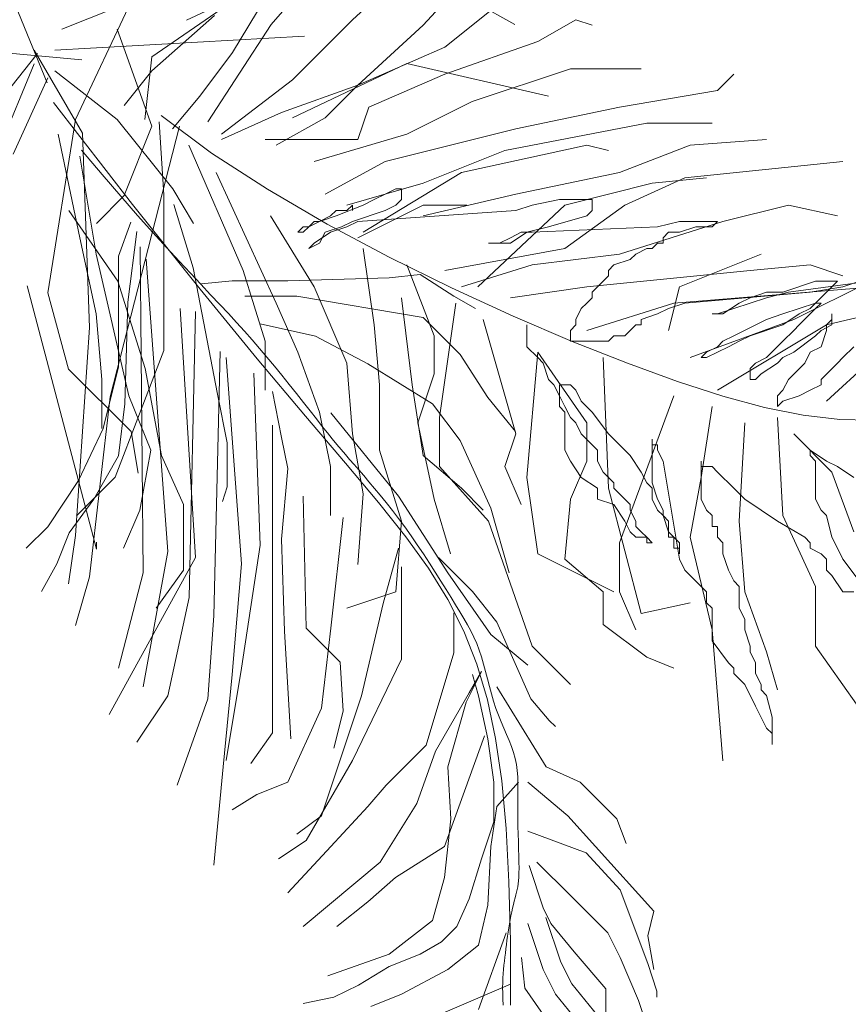
# Model space of a CAD drawing. Units: millimetres. Extents: x 595116 to 630915, y 909473 to 920225.
# Tile 58 of 134: x 629601.67 to 629606.022, y 919290.711 to 919295.882. Entities that reach past the tile are written whole.
import ezdxf

# ---------------------------------------------------------------- set-up
doc = ezdxf.new("R2010")
doc.units = ezdxf.units.MM
doc.layers.add('Dimension', color=3, linetype='Continuous', lineweight=18)
doc.layers.add('L-PLNT', color=85, linetype='Continuous', lineweight=13)
doc.styles.get("Standard").update_dxf_attribs({"font": 'arial.ttf'})
doc.dimstyles.new('ISO-25', dxfattribs={"dimtxt": 9, "dimasz": 6, "dimexe": 1.25, "dimexo": 0.625, "dimtad": 1, "dimlunit": 4, "dimtxsty": 'Standard', "dimcen": 2.5, "dimadec": 0, "dimazin": 0, "dimtfac": 1, "dimtmove": 0, "dimatfit": 3, "dimfxl": 1, "dimarcsym": 0})

# ---------------------------------------------------------------- blocks, each defined once
blk = doc.blocks.new('A$C4FB75ABC')
for p, q in [((2.6324, 2.4053), (2.7073, 2.2214)), ((3.0207, 2.3031), (3.1093, 2.4053)), ((3.1344, 2.3096), (3.2259, 2.3934)), ((3.2335, 2.302), (3.3174, 2.3934)), ((2.9022, 2.3089), (3.0036, 2.3566)), ((2.7277, 2.2964), (2.8733, 2.3546)), ((2.8539, 2.2576), (2.9801, 2.3449)), ((2.8248, 2.3352), (2.7471, 2.1703)), ((2.9666, 2.2638), (3.0123, 2.3401)), ((3.264, 2.2715), (3.3403, 2.3324)), ((3.3079, 2.3327), (3.3615, 2.3029)), ((2.8539, 2.2382), (2.9413, 2.3158)), ((2.9321, 2.167), (3.0207, 2.3031)), ((3.0505, 2.2257), (3.1344, 2.3096)), ((3.142, 2.2181), (3.2335, 2.302)), ((3.3937, 2.2791), (3.447, 2.3096)), ((3.447, 2.3096), (3.4699, 2.302)), ((2.8054, 2.2964), (2.8539, 2.1606)), ((2.7559, 2.2536), (2.4852, 2.2785)), ((2.718, 2.2673), (3.0675, 2.2867)), ((3.264, 2.2334), (3.3937, 2.2791)), ((2.6937, 2.2623), (2.4825, 1.9967)), ((2.6889, 2.2673), (2.7568, 2.1509)), ((2.9208, 2.2029), (2.9666, 2.2638)), ((3.142, 2.2181), (3.264, 2.2715)), ((2.6889, 2.2479), (2.6404, 2.1315)), ((2.8442, 2.1703), (2.8539, 2.2576)), ((3.0505, 2.1724), (3.2106, 2.2486)), ((3.2106, 2.2486), (3.4089, 2.2029)), ((2.718, 2.2382), (2.8054, 2.1703)), ((2.8151, 2.1897), (2.8539, 2.2382)), ((3.1572, 2.1876), (3.264, 2.2334)), ((3.3021, 2.1952), (3.4394, 2.241)), ((3.4394, 2.241), (3.5385, 2.241)), ((3.6453, 2.2105), (3.6682, 2.2334)), ((2.7083, 2.2285), (2.6598, 2.1218)), ((2.9513, 2.1495), (3.0505, 2.2257)), ((3.0352, 2.18), (3.142, 2.2181)), ((3.0962, 2.1724), (3.142, 2.2181)), ((3.508, 2.1876), (3.6453, 2.2105)), ((2.7162, 2.1941), (2.8268, 2.0511)), ((2.8827, 2.1571), (2.9208, 2.2029)), ((3.2106, 2.1495), (3.3021, 2.1952)), ((2.9513, 2.1419), (3.0352, 2.18)), ((3.142, 2.1419), (3.1572, 2.1876)), ((3.3631, 2.1571), (3.508, 2.1876)), ((2.7471, 2.1703), (2.7083, 1.9277)), ((2.8054, 2.1703), (2.883, 2.0733)), ((2.864, 2.167), (2.8708, 2.0648)), ((2.9375, 2.1232), (2.8667, 2.1755)), ((3.0276, 2.1343), (3.0962, 2.1724)), ((3.3479, 2.1266), (3.5462, 2.1648)), ((3.5462, 2.1648), (3.6377, 2.1648)), ((2.7225, 2.1495), (2.753, 2.0047)), ((2.7568, 2.1509), (2.7666, 1.8792)), ((2.8927, 2.1606), (2.7957, 1.7822)), ((2.8539, 2.1606), (2.8151, 2.0636)), ((3.081, 2.1114), (3.2106, 2.1495)), ((3.1801, 2.1114), (3.3631, 2.1571)), ((3.0123, 2.1419), (3.142, 2.1419)), ((3.6072, 2.1343), (3.714, 2.1419)), ((2.7555, 2.1274), (2.7844, 2.0931)), ((2.9056, 2.1343), (2.9818, 1.9589)), ((3.0158, 2.0725), (2.9375, 2.1232)), ((3.2335, 2.0809), (3.3479, 2.1266)), ((3.2869, 2.0961), (3.4623, 2.1343)), ((3.4623, 2.1343), (3.4928, 2.1266)), ((3.508, 2.0961), (3.6072, 2.1343)), ((2.753, 2.119), (2.7759, 1.9818)), ((3.0962, 2.0657), (3.1801, 2.1114)), ((3.5996, 2.0885), (3.8207, 2.1114)), ((2.9437, 2.0961), (3.0276, 1.9132)), ((3.1496, 2.0123), (3.2869, 2.0961)), ((3.3631, 2.0657), (3.508, 2.0961)), ((2.7844, 2.0931), (2.8104, 2.0628)), ((3.1267, 2.0504), (3.2335, 2.0809)), ((3.4318, 2.0504), (3.5538, 2.0809)), ((3.5157, 2.0504), (3.5996, 2.0885)), ((3.5538, 2.0809), (3.6301, 2.0885)), ((2.883, 2.0733), (2.9122, 2.0248)), ((3.0992, 2.0238), (3.0158, 2.0725)), ((3.1954, 2.0733), (3.1801, 2.0657)), ((3.203, 2.0733), (3.1954, 2.0733)), ((3.203, 2.058), (3.203, 2.0733)), ((2.8151, 2.0636), (2.7763, 2.0248)), ((2.8104, 2.0628), (2.8339, 2.0359)), ((2.8708, 2.0648), (2.8708, 1.8469)), ((3.1649, 2.058), (3.1496, 2.0504)), ((3.1801, 2.0657), (3.1649, 2.058)), ((3.1954, 2.0504), (3.203, 2.058)), ((3.2335, 2.0352), (3.3631, 2.0657)), ((3.4242, 2.058), (3.386, 2.0504)), ((3.4699, 2.058), (3.4242, 2.058)), ((3.4699, 2.0428), (3.4699, 2.058)), ((2.7378, 2.0428), (2.8064, 1.9437)), ((2.8268, 2.0511), (2.9214, 1.9326)), ((2.8844, 2.0512), (2.9117, 1.9627)), ((3.1039, 2.0352), (3.1115, 2.0428)), ((3.1496, 2.0504), (3.1115, 2.0352)), ((3.1115, 2.0428), (3.1267, 2.0428)), ((3.1267, 2.0428), (3.1344, 2.0504)), ((3.1344, 2.0504), (3.1344, 2.0428)), ((3.1344, 2.0275), (3.1801, 2.0428)), ((3.142, 2.0047), (3.2335, 2.0504)), ((3.3631, 2.0428), (3.142, 2.0275)), ((3.1801, 2.0428), (3.1954, 2.0504)), ((3.2335, 2.0504), (3.2945, 2.0504)), ((3.3098, 1.9361), (3.4318, 2.0504)), ((3.386, 2.0504), (3.3631, 2.0428)), ((3.4318, 1.9894), (3.5157, 2.0504)), ((3.4623, 2.0352), (3.4699, 2.0428)), ((3.6529, 2.0275), (3.7445, 2.0504)), ((3.7445, 2.0504), (3.8131, 2.0352)), ((2.8244, 2.0263), (2.8071, 1.979)), ((2.8339, 2.0359), (2.8551, 2.0121)), ((3.02, 2.0352), (3.081, 1.9361)), ((3.0734, 2.0199), (3.081, 2.0275)), ((3.0886, 2.0275), (3.0734, 2.0199)), ((3.081, 2.0275), (3.0886, 2.0275)), ((3.1115, 2.0352), (3.0886, 2.0275)), ((3.0886, 2.0275), (3.1039, 2.0352)), ((3.1191, 2.0199), (3.1344, 2.0275)), ((3.142, 2.0275), (3.1267, 2.0199)), ((3.4089, 2.0199), (3.4623, 2.0352)), ((3.508, 1.9818), (3.6529, 2.0275)), ((3.5919, 2.0275), (3.5614, 2.0199)), ((3.6453, 2.0275), (3.5919, 2.0275)), ((3.6377, 2.0199), (3.6453, 2.0275)), ((2.833, 2.0134), (2.8201, 1.9144)), ((2.8551, 2.0121), (2.8744, 1.9909)), ((3.0581, 2.0123), (3.0657, 2.0199)), ((3.0657, 2.0123), (3.0581, 2.0123)), ((3.0734, 2.0199), (3.0657, 2.0123)), ((3.0657, 2.0199), (3.0734, 2.0199)), ((3.1039, 2.0123), (3.081, 1.9971)), ((3.0886, 1.9971), (3.0962, 2.0123)), ((3.0962, 2.0123), (3.1191, 2.0199)), ((3.1858, 1.9776), (3.0992, 2.0238)), ((3.1267, 2.0199), (3.1039, 2.0123)), ((3.3708, 2.0123), (3.3555, 2.0047)), ((3.3555, 1.9971), (3.3784, 2.0123)), ((3.386, 2.0123), (3.3708, 2.0123)), ((3.3784, 2.0123), (3.4089, 2.0199)), ((3.5614, 2.0199), (3.386, 2.0123)), ((3.5691, 2.0047), (3.5767, 2.0123)), ((3.5767, 2.0123), (3.5919, 2.0123)), ((3.5919, 2.0123), (3.6148, 2.0199)), ((3.6148, 2.0199), (3.6377, 2.0199)), ((2.753, 2.0047), (2.7759, 1.898)), ((3.3555, 2.0047), (3.3403, 1.9971)), ((3.5691, 1.9971), (3.5691, 2.0047)), ((2.8373, 1.9919), (2.8416, 1.5357)), ((2.8744, 1.9909), (2.8918, 1.9721)), ((3.081, 1.9971), (3.0734, 1.9894)), ((3.0734, 1.9894), (3.0886, 1.9971)), ((3.1496, 1.9894), (3.1649, 1.8827)), ((3.264, 1.9589), (3.4318, 1.9894)), ((3.3403, 1.9971), (3.325, 1.9971)), ((3.325, 1.9971), (3.3555, 1.9971)), ((3.5309, 1.9818), (3.5462, 1.9894)), ((3.5462, 1.9894), (3.5538, 1.9894)), ((3.5538, 1.9894), (3.5614, 1.9971)), ((3.5614, 1.9971), (3.5691, 1.9971)), ((2.7759, 1.9818), (2.8217, 1.7836)), ((2.8071, 1.979), (2.8071, 1.9015)), ((2.8459, 1.9747), (2.876, 1.5659)), ((2.8918, 1.9721), (2.9078, 1.955)), ((3.2732, 1.9345), (3.1858, 1.9776)), ((3.386, 1.9666), (3.508, 1.9818)), ((3.5004, 1.9666), (3.5233, 1.9742)), ((3.5233, 1.9742), (3.5309, 1.9818)), ((3.5919, 1.9361), (3.7063, 1.9818)), ((2.9117, 1.9627), (2.9458, 1.7856)), ((2.9818, 1.9589), (3.0123, 1.8599)), ((3.2106, 1.9666), (3.2488, 1.8675)), ((3.2869, 1.9361), (3.386, 1.9666)), ((3.4623, 1.9361), (3.6911, 1.9589)), ((3.4928, 1.9589), (3.5004, 1.9666)), ((3.4928, 1.9513), (3.4928, 1.9589)), ((3.6911, 1.9589), (3.775, 1.9666)), ((3.7521, 1.8903), (3.8894, 1.9589)), ((3.775, 1.9666), (3.8207, 1.9513)), ((2.8064, 1.9437), (2.8446, 1.8217)), ((2.9078, 1.955), (2.9225, 1.9395)), ((2.9234, 1.9402), (2.9664, 1.9445)), ((2.9664, 1.9445), (3.0439, 1.9445)), ((3.0439, 1.9445), (3.186, 1.9488)), ((3.186, 1.9488), (3.2291, 1.9531)), ((3.2291, 1.9531), (3.2764, 1.923)), ((3.4699, 1.9285), (3.4852, 1.9437)), ((3.4852, 1.9437), (3.4928, 1.9513)), ((3.7826, 1.9437), (3.7368, 1.9285)), ((3.7445, 1.9285), (3.9122, 1.9513)), ((3.7826, 1.9132), (3.8131, 1.9437)), ((3.8131, 1.9437), (3.7826, 1.9437)), ((3.7978, 1.8827), (4.0495, 1.9437)), ((3.8665, 1.9513), (3.8207, 1.9361)), ((2.6792, 1.9375), (2.7763, 1.5688)), ((2.9214, 1.9326), (3.0014, 1.8351)), ((2.9225, 1.9395), (2.9361, 1.925)), ((3.081, 1.9361), (3.1267, 1.8294)), ((3.3593, 1.8951), (3.2732, 1.9345)), ((3.3555, 1.9208), (3.4623, 1.9361)), ((3.5767, 1.8751), (3.5919, 1.9361)), ((3.5843, 1.9132), (3.8665, 1.9361)), ((3.8207, 1.9361), (3.775, 1.9285)), ((2.7083, 1.9277), (2.7374, 1.821)), ((2.9361, 1.925), (2.9489, 1.9114)), ((2.9837, 1.923), (3.0569, 1.923)), ((3.0569, 1.923), (3.2334, 1.8929)), ((3.203, 1.9208), (3.2182, 1.7989)), ((3.2764, 1.923), (3.3066, 1.9058)), ((3.4623, 1.9132), (3.4699, 1.9208)), ((3.4699, 1.9208), (3.4699, 1.9285)), ((3.775, 1.9285), (3.5996, 1.9132)), ((3.6453, 1.898), (3.714, 1.9208)), ((3.6911, 1.9208), (3.6758, 1.9132)), ((3.714, 1.9285), (3.6911, 1.9208)), ((3.7368, 1.9285), (3.714, 1.9285)), ((3.714, 1.9208), (3.7445, 1.9285)), ((2.8071, 1.9015), (2.8071, 1.8241)), ((2.8201, 1.9144), (2.8158, 1.7724)), ((2.8933, 1.9058), (2.9148, 1.5573)), ((2.9148, 1.9015), (2.9062, 1.5013)), ((2.9489, 1.9114), (2.9609, 1.8985)), ((3.0276, 1.9132), (3.0581, 1.8446)), ((3.2793, 1.9132), (3.2564, 1.7531)), ((3.447, 1.8903), (3.4547, 1.9056)), ((3.4547, 1.9056), (3.4623, 1.9132)), ((3.4623, 1.8751), (3.5843, 1.9132)), ((3.5767, 1.9056), (3.5614, 1.898)), ((3.5996, 1.9132), (3.5767, 1.9056)), ((3.6758, 1.9132), (3.6529, 1.898)), ((3.7368, 1.898), (3.7826, 1.9132)), ((3.7597, 1.8827), (3.7826, 1.9056)), ((3.775, 1.9056), (3.7597, 1.898)), ((3.7826, 1.9132), (3.775, 1.9056)), ((3.7826, 1.9056), (3.7902, 1.9132)), ((3.7902, 1.9132), (3.7826, 1.9132)), ((2.7759, 1.898), (2.7836, 1.8065)), ((2.9609, 1.8985), (2.9724, 1.8861)), ((3.2334, 1.8929), (3.285, 1.8413)), ((3.3174, 1.8903), (3.3631, 1.7303)), ((3.4421, 1.8597), (3.3593, 1.8951)), ((3.447, 1.8827), (3.447, 1.8903)), ((3.5614, 1.898), (3.5385, 1.8903)), ((3.5385, 1.8903), (3.5385, 1.8827)), ((3.6072, 1.837), (3.7521, 1.8903)), ((3.6529, 1.898), (3.6377, 1.898)), ((3.6377, 1.898), (3.6453, 1.898)), ((3.6682, 1.8675), (3.714, 1.8903)), ((3.714, 1.8903), (3.7368, 1.898)), ((3.7597, 1.898), (3.7368, 1.8827)), ((3.7978, 1.8827), (3.8055, 1.8903)), ((3.8055, 1.8903), (3.8055, 1.898)), ((3.8055, 1.898), (3.8055, 1.8827)), ((2.7666, 1.8792), (2.7471, 1.5882)), ((2.9724, 1.8861), (2.9834, 1.874)), ((2.9834, 1.874), (2.994, 1.862)), ((3.0052, 1.8843), (3.0827, 1.8671)), ((3.1649, 1.8827), (3.1725, 1.7989)), ((3.3784, 1.8827), (3.3784, 1.8522)), ((3.4394, 1.8751), (3.447, 1.8827)), ((3.4394, 1.8599), (3.4394, 1.8751)), ((3.5233, 1.8751), (3.5157, 1.8675)), ((3.5309, 1.8827), (3.5233, 1.8751)), ((3.5385, 1.8827), (3.5309, 1.8827)), ((3.6453, 1.7913), (3.7978, 1.8827)), ((3.7368, 1.8827), (3.6911, 1.8675)), ((3.7368, 1.8599), (3.7521, 1.8751)), ((3.7521, 1.8751), (3.7597, 1.8827)), ((3.7902, 1.8751), (3.7826, 1.8675)), ((3.8055, 1.8827), (3.7902, 1.8751)), ((3.7902, 1.8522), (3.7978, 1.8751)), ((3.7978, 1.8751), (3.7978, 1.8827)), ((2.994, 1.862), (3.0045, 1.8499)), ((3.0123, 1.8599), (3.0123, 1.7913)), ((3.0827, 1.8671), (3.1559, 1.8284)), ((3.2488, 1.8675), (3.2488, 1.8141)), ((3.4928, 1.8599), (3.4394, 1.8599)), ((3.5004, 1.8675), (3.4928, 1.8599)), ((3.5157, 1.8675), (3.5004, 1.8675)), ((3.6453, 1.8522), (3.6529, 1.8599)), ((3.6529, 1.8599), (3.6682, 1.8675)), ((3.6758, 1.8599), (3.6606, 1.8522)), ((3.6911, 1.8675), (3.6758, 1.8599)), ((3.714, 1.837), (3.7368, 1.8599)), ((3.7826, 1.8675), (3.7521, 1.8446)), ((3.7978, 1.776), (3.897, 1.8675)), ((2.8708, 1.8469), (2.8027, 1.6699)), ((3.0045, 1.8499), (3.0149, 1.8377)), ((3.3784, 1.8522), (3.3937, 1.837)), ((3.5192, 1.829), (3.4421, 1.8597)), ((3.6606, 1.8522), (3.6301, 1.837)), ((3.6301, 1.8446), (3.6453, 1.8522)), ((3.775, 1.8446), (3.7902, 1.8522)), ((3.836, 1.8522), (3.8207, 1.837)), ((2.9492, 1.8456), (2.9406, 1.4755)), ((2.9578, 1.837), (2.9794, 1.5486)), ((3.0014, 1.8351), (3.0686, 1.7552)), ((3.0149, 1.8377), (3.0253, 1.8251)), ((3.0581, 1.8446), (3.0886, 1.7608)), ((3.285, 1.8413), (3.3238, 1.781)), ((3.3937, 1.8446), (3.3784, 1.6693)), ((3.3937, 1.8446), (3.4623, 1.7455)), ((3.3937, 1.837), (3.4013, 1.8294)), ((3.4852, 1.837), (3.4928, 1.6541)), ((3.6224, 1.837), (3.6301, 1.8446)), ((3.6301, 1.837), (3.6224, 1.837)), ((3.6987, 1.8294), (3.714, 1.837)), ((3.7368, 1.837), (3.7292, 1.8294)), ((3.7521, 1.8446), (3.7368, 1.837)), ((3.7673, 1.8294), (3.775, 1.8446)), ((3.8207, 1.837), (3.8131, 1.8294)), ((2.7374, 1.821), (2.8248, 1.7337)), ((2.8071, 1.8241), (2.7856, 1.738)), ((2.8446, 1.8217), (2.8674, 1.6998)), ((3.0253, 1.8251), (3.0358, 1.8122)), ((3.1267, 1.8294), (3.1344, 1.7303)), ((3.1559, 1.8284), (3.2463, 1.7724)), ((3.4013, 1.8294), (3.4089, 1.8065)), ((3.5892, 1.8034), (3.5192, 1.829)), ((3.6911, 1.8217), (3.6987, 1.8294)), ((3.6911, 1.8065), (3.6911, 1.8217)), ((3.7292, 1.8294), (3.7063, 1.8141)), ((3.7445, 1.8065), (3.7673, 1.8294)), ((3.8131, 1.8294), (3.7902, 1.8065)), ((2.7836, 1.8065), (2.7836, 1.7379)), ((2.9966, 1.8154), (3.0052, 1.5745)), ((3.0358, 1.8122), (3.0461, 1.7993)), ((3.2488, 1.8141), (3.2259, 1.7455)), ((3.4089, 1.8065), (3.4165, 1.7989)), ((3.6987, 1.8065), (3.6911, 1.8065)), ((3.7063, 1.8141), (3.6987, 1.8065)), ((3.7368, 1.7913), (3.7445, 1.8065)), ((3.7902, 1.8065), (3.7902, 1.7989)), ((3.0461, 1.7993), (3.0562, 1.7866)), ((3.1725, 1.7989), (3.1725, 1.7074)), ((3.2182, 1.7989), (3.2335, 1.6998)), ((3.4165, 1.7989), (3.4242, 1.7836)), ((3.4242, 1.7684), (3.4242, 1.7989)), ((3.4242, 1.7989), (3.4394, 1.7989)), ((3.4394, 1.7989), (3.447, 1.7913)), ((3.447, 1.7913), (3.4547, 1.776)), ((3.6527, 1.7828), (3.5892, 1.8034)), ((3.7292, 1.7836), (3.7368, 1.7913)), ((3.775, 1.7913), (3.7597, 1.7836)), ((3.7902, 1.7989), (3.775, 1.7913)), ((2.7957, 1.7822), (2.7666, 1.53)), ((2.8217, 1.7836), (2.8522, 1.7074)), ((2.9458, 1.7856), (2.9594, 1.7175)), ((3.0224, 1.7896), (3.0353, 1.7251)), ((3.0562, 1.7866), (3.0659, 1.7741)), ((3.3238, 1.781), (3.3625, 1.7337)), ((3.4242, 1.7836), (3.4318, 1.7684)), ((3.5843, 1.7836), (3.508, 1.5778)), ((3.7109, 1.7672), (3.6527, 1.7828)), ((3.7292, 1.7684), (3.7292, 1.7836)), ((3.7597, 1.7836), (3.7368, 1.776)), ((2.8158, 1.7724), (2.8071, 1.6993)), ((3.0659, 1.7741), (3.0752, 1.7623)), ((3.2463, 1.7724), (3.285, 1.7208)), ((3.4318, 1.7608), (3.4242, 1.7684)), ((3.4318, 1.7684), (3.4394, 1.7531)), ((3.4547, 1.776), (3.4699, 1.7608)), ((3.6377, 1.7684), (3.6224, 1.6693)), ((3.7651, 1.7564), (3.7109, 1.7672)), ((3.7368, 1.776), (3.7292, 1.7684)), ((3.0686, 1.7552), (3.1246, 1.6894)), ((3.0752, 1.7623), (3.084, 1.7511)), ((3.084, 1.7511), (3.0921, 1.7408)), ((3.0886, 1.7608), (3.1039, 1.6845)), ((3.1042, 1.7595), (3.1989, 1.6433)), ((3.2564, 1.7531), (3.2564, 1.6845)), ((3.4318, 1.7074), (3.4318, 1.7608)), ((3.4394, 1.7531), (3.447, 1.7455)), ((3.4699, 1.7608), (3.4928, 1.7303)), ((3.7292, 1.7531), (3.7368, 1.6159)), ((3.8165, 1.7504), (3.7651, 1.7564)), ((3.8664, 1.749), (3.8165, 1.7504)), ((2.7856, 1.738), (2.7512, 1.6648)), ((3.0224, 1.7423), (3.0224, 1.312)), ((3.0921, 1.7408), (3.0994, 1.7316)), ((3.2259, 1.7455), (3.2488, 1.6388)), ((3.447, 1.7455), (3.4547, 1.7303)), ((3.4623, 1.7455), (3.4623, 1.6922)), ((3.6834, 1.7455), (3.6758, 1.6083)), ((2.8248, 1.7337), (2.8345, 1.6755)), ((3.0353, 1.7251), (3.0439, 1.682)), ((3.0994, 1.7316), (3.1062, 1.7232)), ((3.1062, 1.7232), (3.1126, 1.7155)), ((3.1344, 1.7303), (3.1496, 1.6464)), ((3.3631, 1.7303), (3.3479, 1.6845)), ((3.4547, 1.7303), (3.4699, 1.715)), ((3.4928, 1.7303), (3.508, 1.715)), ((3.5538, 1.7227), (3.5538, 1.715)), ((3.5538, 1.6617), (3.5538, 1.7227)), ((3.7521, 1.7303), (3.8055, 1.6769)), ((2.9594, 1.7175), (2.9594, 1.6563)), ((3.1126, 1.7155), (3.1186, 1.7083)), ((3.1186, 1.7083), (3.1246, 1.7013)), ((3.285, 1.7208), (3.3281, 1.6261)), ((3.4699, 1.715), (3.4775, 1.7074)), ((3.508, 1.715), (3.5233, 1.6998)), ((3.5538, 1.715), (3.5614, 1.715)), ((3.5614, 1.715), (3.5614, 1.7074)), ((2.8071, 1.6993), (2.7727, 1.639)), ((2.8522, 1.7074), (2.8369, 1.6236)), ((2.8674, 1.6998), (2.8979, 1.6312)), ((3.1246, 1.7013), (3.1305, 1.6944)), ((3.1725, 1.7074), (3.203, 1.6083)), ((3.2335, 1.6998), (3.2869, 1.6541)), ((3.4394, 1.6922), (3.4318, 1.7074)), ((3.4775, 1.7074), (3.4775, 1.6922)), ((3.5233, 1.6998), (3.5385, 1.6769)), ((3.5614, 1.7074), (3.5691, 1.6922)), ((3.775, 1.6998), (3.775, 1.7074)), ((3.775, 1.7074), (3.7978, 1.6922)), ((3.7826, 1.6922), (3.775, 1.6998)), ((3.0439, 1.682), (3.0353, 1.5831)), ((3.1039, 1.6845), (3.1039, 1.6159)), ((3.1246, 1.6894), (3.1709, 1.6342)), ((3.1305, 1.6944), (3.1367, 1.6873)), ((3.1367, 1.6873), (3.1432, 1.6798)), ((3.2564, 1.6845), (3.325, 1.6083)), ((3.3479, 1.6845), (3.3708, 1.6312)), ((3.4547, 1.6693), (3.4394, 1.6922)), ((3.4623, 1.6922), (3.4394, 1.6388)), ((3.4775, 1.6922), (3.4852, 1.6769)), ((3.5691, 1.6922), (3.5919, 1.555)), ((3.6224, 1.6922), (3.6224, 1.6845)), ((3.6224, 1.6388), (3.6224, 1.6922)), ((3.6224, 1.6845), (3.6377, 1.6845)), ((3.6377, 1.6845), (3.6453, 1.6769)), ((3.7826, 1.6388), (3.7826, 1.6922)), ((3.7978, 1.6922), (3.8131, 1.6845)), ((3.8131, 1.6845), (3.836, 1.6693)), ((2.8027, 1.6699), (2.7482, 1.6154)), ((3.1432, 1.6798), (3.1502, 1.6718)), ((3.1502, 1.6718), (3.1576, 1.6632)), ((3.3784, 1.6693), (3.3937, 1.5626)), ((3.4775, 1.6541), (3.4547, 1.6693)), ((3.4852, 1.6769), (3.4928, 1.6693)), ((3.4928, 1.6693), (3.5004, 1.6617)), ((3.5385, 1.6769), (3.5462, 1.6617)), ((3.6224, 1.6693), (3.6072, 1.5855)), ((3.6453, 1.6769), (3.6682, 1.6541)), ((3.8055, 1.6769), (3.836, 1.5931)), ((2.7512, 1.6648), (2.7081, 1.6003)), ((2.9594, 1.6563), (2.9526, 1.6358)), ((3.1576, 1.6632), (3.1654, 1.654)), ((3.1654, 1.654), (3.1735, 1.6443)), ((3.2869, 1.6541), (3.3174, 1.6236)), ((3.4775, 1.6388), (3.4775, 1.6541)), ((3.4928, 1.6541), (3.5385, 1.4787)), ((3.5004, 1.6617), (3.5004, 1.6541)), ((3.5004, 1.6541), (3.5157, 1.6388)), ((3.5462, 1.6617), (3.5538, 1.6541)), ((3.5614, 1.6388), (3.5538, 1.6617)), ((3.5538, 1.6541), (3.5538, 1.6388)), ((3.6682, 1.6541), (3.6834, 1.6388)), ((3.0655, 1.6433), (3.0698, 1.4583)), ((3.1496, 1.6464), (3.142, 1.5473)), ((3.1735, 1.6443), (3.1819, 1.634)), ((3.1989, 1.6433), (3.2678, 1.5357)), ((2.7727, 1.639), (2.7383, 1.5917)), ((2.8979, 1.6312), (2.8979, 1.5397)), ((3.1709, 1.6342), (3.2091, 1.5863)), ((3.1819, 1.634), (3.1904, 1.6232)), ((3.2488, 1.6388), (3.2716, 1.5626)), ((3.3281, 1.6261), (3.3539, 1.5357)), ((3.4394, 1.6388), (3.4318, 1.555)), ((3.5004, 1.6312), (3.4775, 1.6388)), ((3.5157, 1.6083), (3.5004, 1.6312)), ((3.5157, 1.6388), (3.5233, 1.6312)), ((3.5233, 1.6312), (3.5233, 1.6236)), ((3.5538, 1.6388), (3.5614, 1.6236)), ((3.5691, 1.6236), (3.5614, 1.6388)), ((3.6301, 1.6236), (3.6224, 1.6388)), ((3.6834, 1.6388), (3.7292, 1.6083)), ((3.7902, 1.6236), (3.7826, 1.6388)), ((2.8369, 1.6236), (2.8141, 1.5702)), ((3.1214, 1.6132), (3.1042, 1.4583)), ((3.1904, 1.6232), (3.1991, 1.6119)), ((3.1991, 1.6119), (3.2078, 1.6)), ((3.5233, 1.6236), (3.5309, 1.6083)), ((3.5614, 1.6236), (3.5691, 1.6159)), ((3.5691, 1.6159), (3.5691, 1.6236)), ((3.5691, 1.6159), (3.5767, 1.6083)), ((3.5767, 1.5931), (3.5691, 1.6159)), ((3.6377, 1.6159), (3.6301, 1.6236)), ((3.6377, 1.6007), (3.6377, 1.6159)), ((3.7368, 1.6159), (3.7826, 1.5168)), ((3.7978, 1.6159), (3.7902, 1.6236)), ((3.8055, 1.5855), (3.7978, 1.6159)), ((2.7081, 1.6003), (2.678, 1.5702)), ((3.203, 1.6083), (3.1954, 1.5092)), ((3.2078, 1.6), (3.2166, 1.5877)), ((3.325, 1.6083), (3.386, 1.433)), ((3.5233, 1.5931), (3.5157, 1.6083)), ((3.5309, 1.6083), (3.5309, 1.6007)), ((3.5309, 1.6007), (3.5385, 1.5931)), ((3.5767, 1.6083), (3.5767, 1.5855)), ((3.6453, 1.6007), (3.6377, 1.6007)), ((3.6453, 1.5855), (3.6453, 1.6007)), ((3.6758, 1.6083), (3.6834, 1.5092)), ((3.7292, 1.6083), (3.7673, 1.5855)), ((2.7383, 1.5917), (2.721, 1.5486)), ((2.7471, 1.5882), (2.7374, 1.5203)), ((3.2091, 1.5863), (3.241, 1.5422)), ((3.2166, 1.5877), (3.2252, 1.575)), ((3.5309, 1.5855), (3.5233, 1.5931)), ((3.5462, 1.5855), (3.5309, 1.5855)), ((3.5385, 1.5931), (3.5462, 1.5855)), ((3.5462, 1.5855), (3.5462, 1.5778)), ((3.5538, 1.5778), (3.5462, 1.5855)), ((3.5843, 1.5855), (3.5767, 1.5931)), ((3.5767, 1.5855), (3.5843, 1.5855)), ((3.5843, 1.5855), (3.5843, 1.5702)), ((3.5919, 1.5778), (3.5843, 1.5855)), ((3.6072, 1.5855), (3.6377, 1.4559)), ((3.6529, 1.5778), (3.6453, 1.5855)), ((3.7673, 1.5855), (3.775, 1.5778)), ((3.8131, 1.5702), (3.8055, 1.5855)), ((2.7763, 1.5688), (2.7763, 1.5785)), ((3.0052, 1.5745), (2.9794, 1.4023)), ((3.0353, 1.5831), (3.0396, 1.454)), ((3.2252, 1.575), (3.2338, 1.5622)), ((3.508, 1.5778), (3.508, 1.5092)), ((3.5462, 1.5778), (3.5538, 1.5778)), ((3.5919, 1.5626), (3.5919, 1.5778)), ((3.6529, 1.5626), (3.6529, 1.5778)), ((3.775, 1.5778), (3.775, 1.5702)), ((2.9148, 1.5573), (2.7942, 1.3378)), ((2.876, 1.5659), (2.8416, 1.3765)), ((3.1989, 1.5702), (3.1774, 1.4927)), ((3.2338, 1.5622), (3.2421, 1.5493)), ((3.2549, 1.5573), (3.3023, 1.5099)), ((3.3937, 1.5626), (3.4852, 1.5168)), ((3.5843, 1.5702), (3.5919, 1.5702)), ((3.5919, 1.5702), (3.5919, 1.5626)), ((3.6606, 1.5397), (3.6529, 1.5626)), ((3.775, 1.5702), (3.7902, 1.5626)), ((3.7902, 1.5626), (3.7978, 1.555)), ((3.8207, 1.555), (3.8131, 1.5702)), ((2.721, 1.5486), (2.6995, 1.5099)), ((2.9794, 1.5486), (2.9664, 1.3937)), ((3.2032, 1.5443), (3.2032, 1.4152)), ((3.2421, 1.5493), (3.2503, 1.5367)), ((3.4318, 1.555), (3.4852, 1.5092)), ((3.5919, 1.555), (3.5996, 1.5397)), ((3.7978, 1.555), (3.7978, 1.5397)), ((3.8436, 1.5245), (3.8207, 1.555)), ((2.7666, 1.53), (2.7471, 1.462)), ((2.8416, 1.5357), (2.8071, 1.4023)), ((2.8979, 1.5397), (2.8598, 1.4864)), ((3.241, 1.5422), (3.2678, 1.4987)), ((3.2503, 1.5367), (3.258, 1.5243)), ((3.2678, 1.5357), (3.3281, 1.4497)), ((3.5996, 1.5397), (3.6301, 1.5092)), ((3.6682, 1.5245), (3.6606, 1.5397)), ((3.7978, 1.5397), (3.8055, 1.5321)), ((3.8055, 1.5321), (3.8207, 1.5092)), ((3.258, 1.5243), (3.2655, 1.5125)), ((3.4852, 1.5168), (3.5004, 1.5092)), ((3.6758, 1.5168), (3.6682, 1.5245)), ((3.6758, 1.4864), (3.6758, 1.5168)), ((3.7826, 1.5168), (3.7826, 1.433)), ((3.1954, 1.5092), (3.1267, 1.4864)), ((3.2655, 1.5125), (3.2724, 1.5013)), ((3.3023, 1.5099), (3.3367, 1.4669)), ((3.4852, 1.5092), (3.4852, 1.4635)), ((3.508, 1.5092), (3.5309, 1.4559)), ((3.6301, 1.5092), (3.6301, 1.494)), ((3.6834, 1.5092), (3.714, 1.4254)), ((3.8207, 1.5092), (3.836, 1.5092)), ((2.9062, 1.5013), (2.876, 1.3636)), ((3.1774, 1.4927), (3.1473, 1.3636)), ((3.2678, 1.4987), (3.2902, 1.4543)), ((3.2724, 1.5013), (3.2789, 1.491)), ((3.2789, 1.491), (3.2849, 1.4813)), ((3.5385, 1.4787), (3.6072, 1.494)), ((3.6301, 1.494), (3.6377, 1.4864)), ((2.9406, 1.4755), (2.932, 1.3593)), ((3.2764, 1.4798), (3.2764, 1.4239)), ((3.2849, 1.4813), (3.2904, 1.4721)), ((3.6377, 1.4864), (3.6377, 1.4406)), ((3.6834, 1.4711), (3.6758, 1.4864)), ((3.2904, 1.4721), (3.2955, 1.4632)), ((3.2955, 1.4632), (3.3002, 1.4545)), ((3.3367, 1.4669), (3.3841, 1.3593)), ((3.4852, 1.4635), (3.5462, 1.4178)), ((3.6834, 1.4559), (3.6834, 1.4711)), ((3.0396, 1.454), (3.0483, 1.3034)), ((3.0698, 1.4583), (3.1171, 1.4109)), ((3.1042, 1.4583), (3.0913, 1.3464)), ((3.2902, 1.4543), (3.3086, 1.4079)), ((3.3002, 1.4545), (3.3045, 1.4458)), ((3.3281, 1.4497), (3.3798, 1.4066)), ((3.6377, 1.4559), (3.6529, 1.2729)), ((3.6911, 1.433), (3.6834, 1.4559)), ((3.3045, 1.4458), (3.3084, 1.437)), ((3.3084, 1.437), (3.3119, 1.4278)), ((3.386, 1.433), (3.4394, 1.3796)), ((3.6377, 1.4406), (3.6606, 1.4101)), ((3.6911, 1.4254), (3.6911, 1.433)), ((3.7826, 1.433), (3.8741, 1.3034)), ((3.2764, 1.4239), (3.2377, 1.2948)), ((3.3119, 1.4278), (3.3151, 1.4181)), ((3.6987, 1.4101), (3.6911, 1.4254)), ((3.714, 1.4254), (3.7292, 1.372)), ((3.1171, 1.4109), (3.1214, 1.3421)), ((3.2032, 1.4152), (3.1344, 1.2732)), ((3.3086, 1.4079), (3.3233, 1.3583)), ((3.3151, 1.4181), (3.3181, 1.4081)), ((3.3181, 1.4081), (3.3209, 1.3978)), ((3.5462, 1.4178), (3.5843, 1.4025)), ((3.6606, 1.4101), (3.6682, 1.4025)), ((3.6987, 1.3949), (3.6987, 1.4101)), ((2.9664, 1.3937), (2.9535, 1.2646)), ((2.9794, 1.4023), (2.9578, 1.2732)), ((3.2937, 1.355), (3.3152, 1.398)), ((3.298, 1.3679), (3.3152, 1.398)), ((3.3023, 1.3937), (3.3109, 1.3636)), ((3.3209, 1.3978), (3.3236, 1.3873)), ((3.6682, 1.4025), (3.6682, 1.3949)), ((3.6682, 1.3949), (3.6834, 1.3796)), ((3.7063, 1.3796), (3.6987, 1.3949)), ((3.3236, 1.3873), (3.3263, 1.3768)), ((3.6834, 1.3796), (3.6987, 1.3492)), ((3.7063, 1.372), (3.7063, 1.3796)), ((3.2506, 1.2861), (3.298, 1.3679)), ((3.3263, 1.3768), (3.3291, 1.3664)), ((3.3291, 1.3664), (3.332, 1.3561)), ((3.3367, 1.3765), (3.4056, 1.2646)), ((3.714, 1.3644), (3.7063, 1.372)), ((3.7216, 1.3339), (3.714, 1.3644)), ((2.876, 1.3636), (2.833, 1.2991)), ((2.932, 1.3593), (2.889, 1.2388)), ((3.1473, 1.3636), (3.0913, 1.1958)), ((3.2678, 1.2646), (3.2937, 1.355)), ((3.3109, 1.3636), (3.3238, 1.3034)), ((3.3233, 1.3583), (3.3348, 1.3042)), ((3.332, 1.3561), (3.3352, 1.3462)), ((3.3841, 1.3593), (3.4099, 1.3292)), ((3.0913, 1.3464), (3.0439, 1.2431)), ((3.1214, 1.3421), (3.1085, 1.2905)), ((3.3352, 1.3462), (3.3388, 1.3366)), ((3.3388, 1.3366), (3.3425, 1.3274)), ((3.6987, 1.3492), (3.714, 1.3187)), ((3.3425, 1.3274), (3.3463, 1.3185)), ((3.4099, 1.3292), (3.4185, 1.3206)), ((3.7216, 1.2958), (3.7216, 1.3339)), ((3.0224, 1.312), (2.9923, 1.2689)), ((3.3463, 1.3185), (3.3501, 1.3098)), ((3.3501, 1.3098), (3.3537, 1.3013)), ((3.714, 1.3187), (3.7216, 1.311)), ((3.7216, 1.311), (3.7216, 1.2958)), ((3.3195, 1.3077), (3.2635, 1.1527)), ((3.3238, 1.3034), (3.3324, 1.2431)), ((3.3348, 1.3042), (3.3434, 1.2446)), ((3.3537, 1.3013), (3.357, 1.2929)), ((3.2377, 1.2948), (3.1817, 1.2388)), ((3.2248, 1.213), (3.2506, 1.2861)), ((3.357, 1.2929), (3.3598, 1.2846)), ((3.3598, 1.2846), (3.3622, 1.2762)), ((3.1344, 1.2732), (3.0698, 1.1614)), ((3.3622, 1.2762), (3.3639, 1.2677)), ((3.3639, 1.2677), (3.365, 1.2592)), ((2.9535, 1.2646), (2.9406, 1.1269)), ((3.2721, 1.1915), (3.2678, 1.2646)), ((3.365, 1.2592), (3.3657, 1.2504)), ((3.4056, 1.2646), (3.453, 1.2431)), ((3.0439, 1.2431), (3.0009, 1.2259)), ((3.3324, 1.2431), (3.3324, 1.1872)), ((3.3367, 1.2087), (3.3669, 1.2431)), ((3.3434, 1.2446), (3.3495, 1.1781)), ((3.3657, 1.2504), (3.366, 1.2415)), ((3.366, 1.2415), (3.366, 1.2322)), ((3.3798, 1.2431), (3.4357, 1.1958)), ((3.453, 1.2431), (3.5046, 1.1915)), ((3.1817, 1.2388), (3.1559, 1.2087)), ((3.366, 1.2322), (3.366, 1.2227)), ((3.0009, 1.2259), (2.9664, 1.2044)), ((3.1731, 1.1312), (3.2248, 1.213)), ((3.366, 1.2227), (3.3658, 1.2129)), ((3.3658, 1.2129), (3.3658, 1.2027)), ((3.1559, 1.2087), (3.1042, 1.1527)), ((3.3281, 1.1527), (3.3367, 1.2087)), ((3.3658, 1.2027), (3.3658, 1.1921)), ((3.0913, 1.1958), (3.0569, 1.17)), ((3.2635, 1.1097), (3.2721, 1.1915)), ((3.3324, 1.1872), (3.3152, 1.1355)), ((3.3658, 1.1921), (3.366, 1.1812)), ((3.4357, 1.1958), (3.4745, 1.1527)), ((3.5046, 1.1915), (3.5175, 1.1571)), ((3.3495, 1.1781), (3.3535, 1.1037)), ((3.366, 1.1812), (3.3663, 1.1704)), ((3.3798, 1.1743), (3.4616, 1.1441)), ((3.0698, 1.1614), (3.031, 1.1355)), ((3.3663, 1.1704), (3.3667, 1.1597)), ((3.3667, 1.1597), (3.367, 1.1494)), ((3.1042, 1.1527), (3.0439, 1.0882)), ((3.2635, 1.1527), (3.1946, 1.1097)), ((3.3238, 1.071), (3.3281, 1.1527)), ((3.367, 1.1494), (3.3673, 1.1397)), ((3.4616, 1.1441), (3.5089, 1.0925)), ((3.4745, 1.1527), (3.5563, 1.0624)), ((3.0655, 1.0409), (3.1731, 1.1312)), ((3.3152, 1.1355), (3.298, 1.0796)), ((3.3673, 1.1397), (3.3675, 1.1308)), ((3.3675, 1.1308), (3.3676, 1.1228)), ((3.3927, 1.1312), (3.44, 1.0839)), ((3.3675, 1.116), (3.3672, 1.1101)), ((3.3676, 1.1228), (3.3675, 1.116)), ((3.3816, 1.1261), (3.4013, 1.0669)), ((3.1946, 1.1097), (3.1559, 1.0753)), ((3.2463, 1.0495), (3.2635, 1.1097)), ((3.3535, 1.1037), (3.3557, 1.0207)), ((3.3668, 1.1051), (3.3663, 1.1006)), ((3.3672, 1.1101), (3.3668, 1.1051)), ((3.364, 1.0891), (3.3631, 1.0852)), ((3.3649, 1.0928), (3.364, 1.0891)), ((3.3657, 1.0966), (3.3649, 1.0928)), ((3.3663, 1.1006), (3.3657, 1.0966)), ((3.5089, 1.0925), (3.5477, 0.9892)), ((3.1559, 1.0753), (3.1128, 1.0409)), ((3.298, 1.0796), (3.2807, 1.0409)), ((3.3609, 1.0765), (3.3598, 1.0717)), ((3.362, 1.081), (3.3609, 1.0765)), ((3.3631, 1.0852), (3.362, 1.081)), ((3.44, 1.0839), (3.4917, 1.0323)), ((3.3109, 1.015), (3.3238, 1.071)), ((3.3574, 1.0614), (3.3563, 1.056)), ((3.3586, 1.0667), (3.3574, 1.0614)), ((3.3598, 1.0717), (3.3586, 1.0667)), ((3.4013, 1.0669), (3.4121, 1.0454)), ((3.5563, 1.0624), (3.5477, 1.028)), ((3.186, 1.0021), (3.2463, 1.0495)), ((3.3551, 1.0505), (3.3541, 1.0448)), ((3.3563, 1.056), (3.3551, 1.0505)), ((3.4053, 1.0537), (3.4263, 0.991)), ((3.2807, 1.0409), (3.2592, 1.0193)), ((3.3531, 1.039), (3.3522, 1.0332)), ((3.3541, 1.0448), (3.3531, 1.039)), ((3.3798, 1.0452), (3.4013, 0.9806)), ((3.4121, 1.0454), (3.4447, 1.0056)), ((3.3496, 1.0323), (3.3109, 0.9247)), ((3.3506, 1.0215), (3.3499, 1.0156)), ((3.3514, 1.0274), (3.3506, 1.0215)), ((3.3522, 1.0332), (3.3514, 1.0274)), ((3.3557, 1.0207), (3.3558, 0.9307)), ((3.4917, 1.0323), (3.5089, 0.9978)), ((3.5477, 1.028), (3.5563, 0.9806)), ((3.2592, 1.0193), (3.2291, 1.0021)), ((3.2678, 0.9806), (3.3109, 1.015)), ((3.3492, 1.0097), (3.3485, 1.0039)), ((3.3499, 1.0156), (3.3492, 1.0097)), ((3.0999, 0.972), (3.186, 1.0021)), ((3.2291, 1.0021), (3.186, 0.9849)), ((3.3471, 0.9925), (3.3465, 0.9868)), ((3.3478, 0.9982), (3.3471, 0.9925)), ((3.3485, 1.0039), (3.3478, 0.9982)), ((3.3712, 0.9978), (3.3755, 0.9548)), ((3.4447, 1.0056), (3.4889, 0.9539)), ((3.5089, 0.9978), (3.5348, 0.9376)), ((3.186, 0.9849), (3.143, 0.9591)), ((3.2032, 0.9462), (3.2678, 0.9806)), ((3.3459, 0.981), (3.3454, 0.9751)), ((3.3465, 0.9868), (3.3459, 0.981)), ((3.4013, 0.9806), (3.4185, 0.9462)), ((3.4263, 0.991), (3.4413, 0.9609)), ((3.5477, 0.9892), (3.5606, 0.9505)), ((3.345, 0.9689), (3.3447, 0.9623)), ((3.3454, 0.9751), (3.345, 0.9689)), ((3.143, 0.9591), (3.1085, 0.9419)), ((3.3555, 0.9604), (3.142, 0.8689)), ((3.3447, 0.9623), (3.3446, 0.9554)), ((3.3446, 0.9554), (3.3447, 0.9479)), ((3.3755, 0.9548), (3.4056, 0.9118)), ((3.4413, 0.9609), (3.4779, 0.9162)), ((3.4889, 0.9539), (3.4889, 0.8899)), ((3.1085, 0.9419), (3.0655, 0.9333)), ((3.1602, 0.929), (3.2032, 0.9462)), ((3.3447, 0.9479), (3.3449, 0.9399)), ((3.3449, 0.9399), (3.3453, 0.931)), ((3.4185, 0.9462), (3.4573, 0.8989)), ((3.5348, 0.9376), (3.5735, 0.8214)), ((3.5606, 0.9505), (3.5606, 0.9419))]:
    blk.add_line(p, q)
blk = doc.blocks.new('*D210')
at = {"layer": 'Defpoints', "color": 0, "transparency": 16777216}
for p in [(629586.2273, 919310.1229), (629593.9463, 919310.1229), (629586.2273, 919258.6624)]:
    blk.add_point(p, dxfattribs=at)
at = {"layer": 'Dimension', "color": 0, "lineweight": -2, "transparency": 16777216}
for p, q in [((629593.9463, 919310.1229), (629593.9463, 919449.6901)), ((629586.8523, 919310.1229), (629595.1963, 919310.1229)), ((629593.9463, 919264.6624), (629593.9463, 919304.1229)), ((629586.8523, 919258.6624), (629595.1963, 919258.6624))]:
    blk.add_line(p, q, dxfattribs=at)
at = {"layer": 'Dimension', "color": 0, "transparency": 16777216}
for points in [[(629592.9463, 919304.1229), (629594.9463, 919304.1229), (629593.9463, 919310.1229)], [(629592.9463, 919264.6624), (629594.9463, 919264.6624), (629593.9463, 919258.6624)]]:
    blk.add_solid(points, dxfattribs=at)
at = {"layer": 'Dimension', "color": 0, "transparency": 16777216, "insert": (629588.6617, 919382.9065), "char_height": 9, "attachment_point": 5, "rotation": 90}
blk.add_mtext('CANOPY 4\'-3 1/2" TYP.', dxfattribs=at)
blk = doc.blocks.new('*D216')
at = {"layer": 'Defpoints', "color": 0, "transparency": 16777216}
for p in [(629743.5408, 919411.9276), (629505.0408, 919411.8279), (629743.5408, 918832.3776)]:
    blk.add_point(p, dxfattribs=at)
at = {"layer": 'Dimension', "color": 0, "lineweight": -2, "transparency": 16777216}
for p, q in [((629743.5408, 919411.3026), (629743.5408, 918831.1276)), ((629505.0408, 919411.2029), (629505.0408, 918831.1276)), ((629511.0408, 918832.3776), (629737.5408, 918832.3776))]:
    blk.add_line(p, q, dxfattribs=at)
at = {"layer": 'Dimension', "color": 0, "transparency": 16777216}
for points in [[(629511.0408, 918833.3776), (629511.0408, 918831.3776), (629505.0408, 918832.3776)], [(629737.5408, 918833.3776), (629737.5408, 918831.3776), (629743.5408, 918832.3776)]]:
    blk.add_solid(points, dxfattribs=at)
at = {"layer": 'Dimension', "color": 0, "transparency": 16777216, "insert": (629624.2908, 918837.656), "char_height": 9, "attachment_point": 5}
blk.add_mtext('19\'-10 1/2"', dxfattribs=at)

msp = doc.modelspace()

# ---------------------------------------------------------------- block references
at = {"layer": 'L-PLNT', "xscale": 3.753413438031968, "yscale": 3.753413438031968, "zscale": 3.753413438031968}
msp.add_blockref('A$C4FB75ABC', (629591.6528, 919287.2124), dxfattribs=at)

# ---------------------------------------------------------------- dimensions: what is measured, and where the dimension line sits
at = {"layer": 'Dimension'}
dim = msp.add_linear_dim(base=(629593.9463, 919310.1229), p1=(629586.2273, 919258.6624), p2=(629586.2273, 919310.1229), angle=90, text='CANOPY <> TYP.', dimstyle='ISO-25', override={"dimdec": 1, "dimlfac": 1, "dimrnd": 0, "dimzin": 1, "dimdsep": 46, "dimlunit": 4, "dimfrac": 2}, dxfattribs=at)
dim.commit()
dim.dimension.update_dxf_attribs({"geometry": '*D210', "text_midpoint": (629588.6617, 919382.9065)})
dim = msp.add_linear_dim(base=(629743.5408, 918832.3776), p1=(629505.0408, 919411.8279), p2=(629743.5408, 919411.9276), dimstyle='ISO-25', override={"dimdec": 1, "dimlfac": 1, "dimrnd": 0, "dimzin": 1, "dimdsep": 46, "dimlunit": 4, "dimfrac": 2}, dxfattribs=at)
dim.commit()
dim.dimension.update_dxf_attribs({"geometry": '*D216', "text_midpoint": (629624.2908, 918837.656)})

doc.saveas('drawing.dxf')
